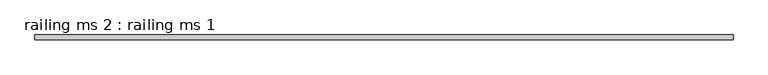
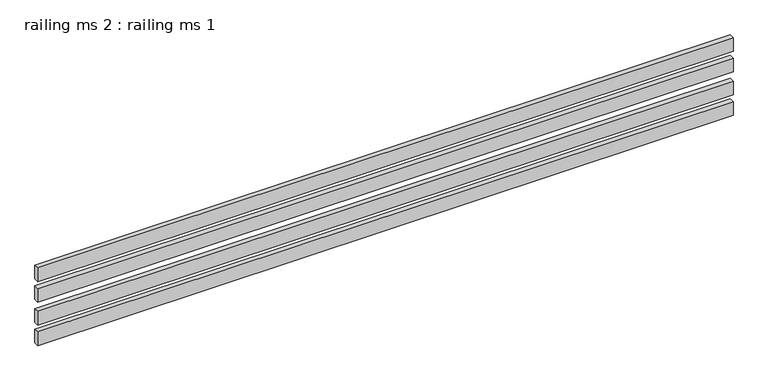
"""IFC4 building model written with IfcOpenShell, lengths in millimetres: proxy geometry, railing ms 2 : railing ms 1."""

from ifc_helpers import new_model, si_unit, frame, origin, place, context, project, spatial, polyline, outline, extrude, source, transform, mapped, element, save


def railing_ms_2_railing_ms_1_4ed16cdf(model_context):
    return source(origin(), model_context, "Body", "SweptSolid", [
        extrude(outline(polyline([(-15346.729089, -4511.3468048), (-15346.729089, -4536.7468048), (-19004.329089, -4536.7468048), (-19004.329089, -4511.3468048), (-15346.729089, -4511.3468048)])), frame((0.0, 0.0, 7052.1286522), z_axis=(0.0, 0.0, 1.0), x_axis=(1.0, 0.0, 0.0)), (0.0, 0.0, 1.0), 76.2),
        extrude(outline(polyline([(-15346.729089, -4511.3468048), (-15346.729089, -4536.7468048), (-19004.329089, -4536.7468048), (-19004.329089, -4511.3468048), (-15346.729089, -4511.3468048)])), frame((0.0, 0.0, 7166.4286522), z_axis=(0.0, 0.0, 1.0), x_axis=(1.0, 0.0, 0.0)), (0.0, 0.0, 1.0), 76.2),
        extrude(outline(polyline([(-15346.729089, -4511.3468048), (-15346.729089, -4536.7468048), (-19004.329089, -4536.7468048), (-19004.329089, -4511.3468048), (-15346.729089, -4511.3468048)])), frame((0.0, 0.0, 7293.4286522), z_axis=(0.0, 0.0, 1.0), x_axis=(1.0, 0.0, 0.0)), (0.0, 0.0, 1.0), 76.2),
        extrude(outline(polyline([(-15346.729089, -4511.3468048), (-15346.729089, -4536.7468048), (-19004.329089, -4536.7468048), (-19004.329089, -4511.3468048), (-15346.729089, -4511.3468048)])), frame((0.0, 0.0, 7407.7286522), z_axis=(0.0, 0.0, 1.0), x_axis=(1.0, 0.0, 0.0)), (0.0, 0.0, 1.0), 76.2),
    ])


if __name__ == "__main__":
    model = new_model("IFC4")
    model_context = context("Model", 3, world=origin())
    ifc_project = project(units=[si_unit("LENGTHUNIT", "METRE", prefix="MILLI")], contexts=[model_context])
    site = spatial("IfcSite", under=ifc_project)
    building = spatial("IfcBuilding", under=site)
    placement = place(None, origin())
    railing_ms_2_railing_ms_1_shape = railing_ms_2_railing_ms_1_4ed16cdf(model_context)
    element("IfcBuildingElementProxy", 1, Name="railing ms 2 : railing ms 1", ObjectType="railing ms 2 : railing ms 1", at=placement, inside=building, context=model_context, shape_type="MappedRepresentation", body=[
        mapped(railing_ms_2_railing_ms_1_shape, transform((0.0, 0.0, 0.0), x_axis=(1.0, 0.0, 0.0), y_axis=(0.0, 1.0, 0.0), z_axis=(0.0, 0.0, 1.0))),
    ])
    save(model, "model.ifc")
